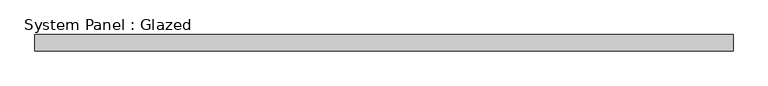
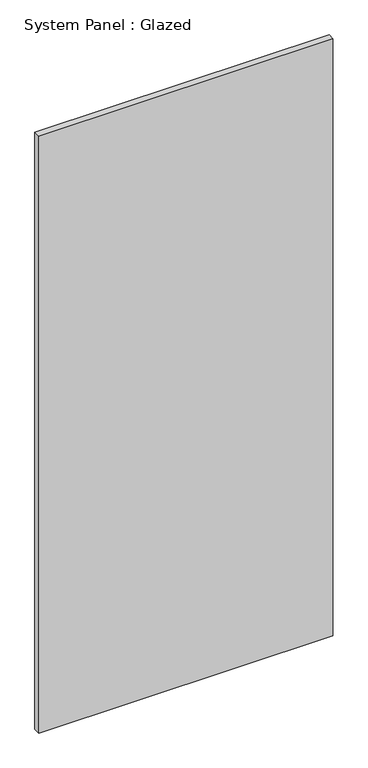
"""IFC4 building model written with IfcOpenShell, lengths in millimetres: plate geometry, System Panel : Glazed."""

from ifc_helpers import new_model, si_unit, origin, origin_with_axes, place, context, project, spatial, polyline, outline, extrude, source, transform, mapped, element, save


def system_panel_glazed_c5a9eb28(model_context):
    return source(origin(), model_context, "Body", "SweptSolid", [
        extrude(outline(polyline([(546.1, 19.05), (-546.1, 19.05), (-546.1, 44.45), (546.1, 44.45), (546.1, 19.05)])), origin_with_axes(), (0.0, 0.0, 1.0), 2343.15),
    ])


if __name__ == "__main__":
    model = new_model("IFC4")
    model_context = context("Model", 3, world=origin())
    ifc_project = project(units=[si_unit("LENGTHUNIT", "METRE", prefix="MILLI")], contexts=[model_context])
    site = spatial("IfcSite", under=ifc_project)
    building = spatial("IfcBuilding", under=site)
    placement = place(None, origin())
    system_panel_glazed_shape = system_panel_glazed_c5a9eb28(model_context)
    element("IfcPlate", 1, ObjectType="System Panel : Glazed", at=placement, inside=building, context=model_context, shape_type="MappedRepresentation", body=[
        mapped(system_panel_glazed_shape, transform((0.0, 0.0, 0.0), x_axis=(1.0, 0.0, 0.0), y_axis=(0.0, 1.0, 0.0), z_axis=(0.0, 0.0, 1.0))),
    ])
    save(model, "model.ifc")

# Revit data of these elements
# Type "System Panel : Glazed"
#   Construction Type Id = "GSP4R"
#   Analytic Construction = "1/8 in Pilkington single glazing"
#   Visual Light Transmittance = 0.9
#   Solar Heat Gain Coefficient = 0.86
#   Heat Transfer Coefficient (U) = 1.18115 BTU/(h·ft²·°F)
#   Define Thermal Properties by = 1
# Element 1 (IfcPlate, "System Panel : Glazed")
#   Materials on its faces: "Glass"
# Materials
#   "Glass": class "Glass", colour RGB 0 128 192, transparency 0.75, Description = "Soda Lime Glass", Cost = 0
